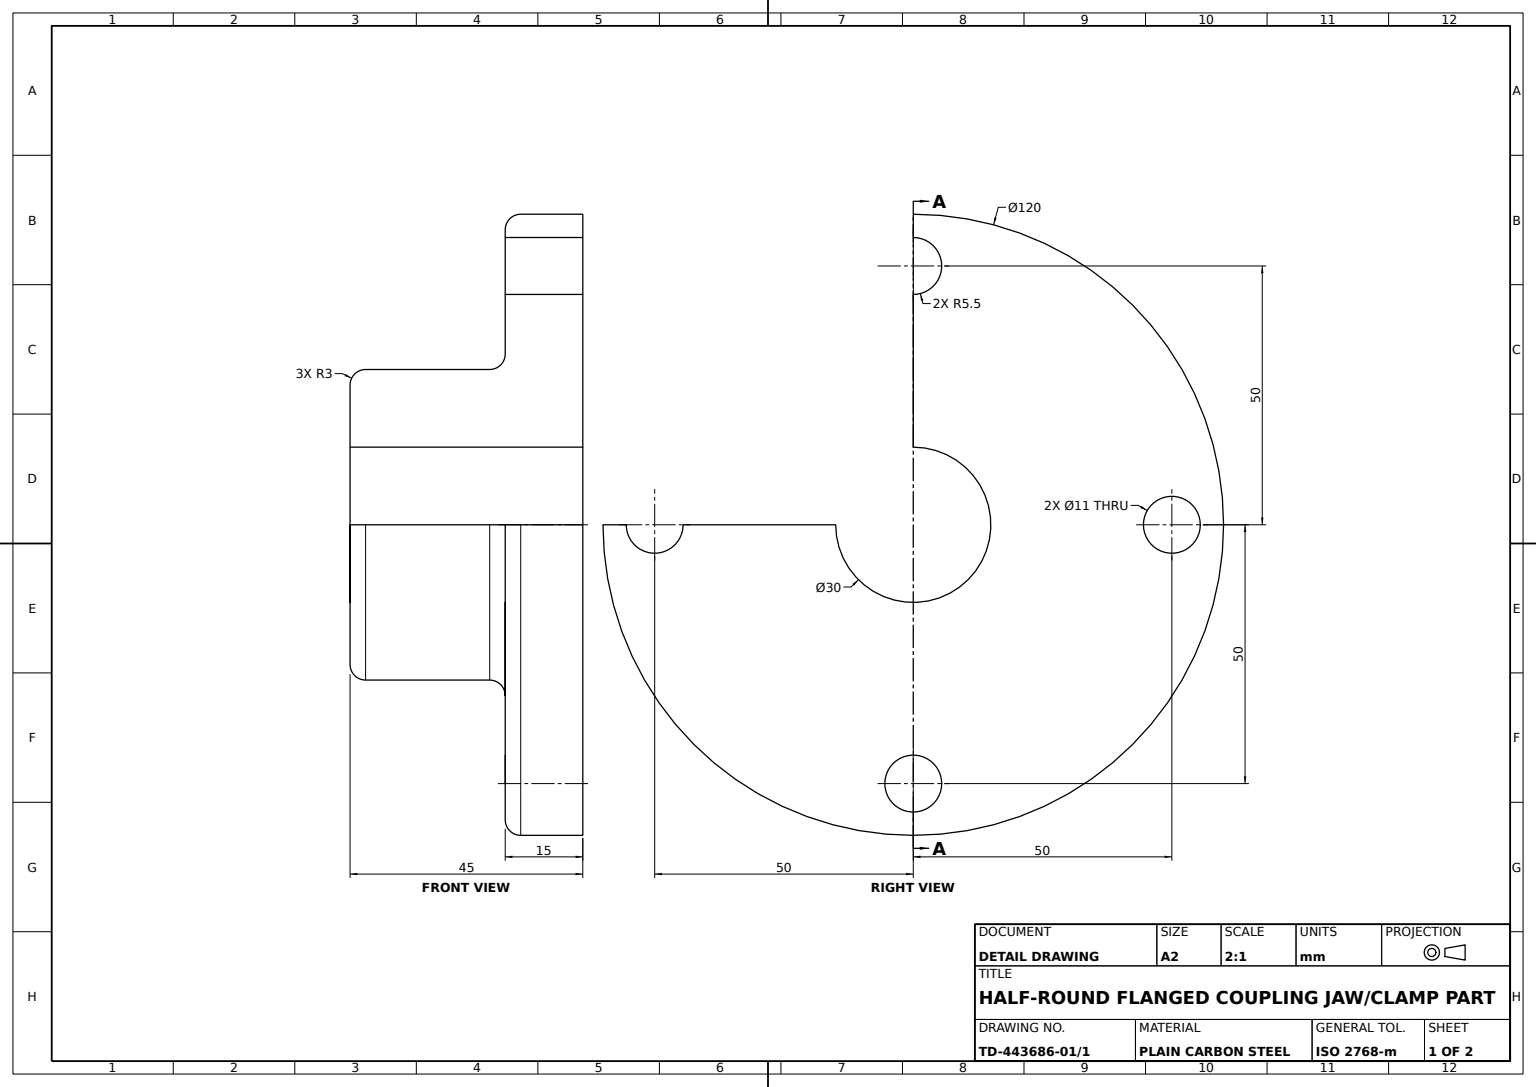
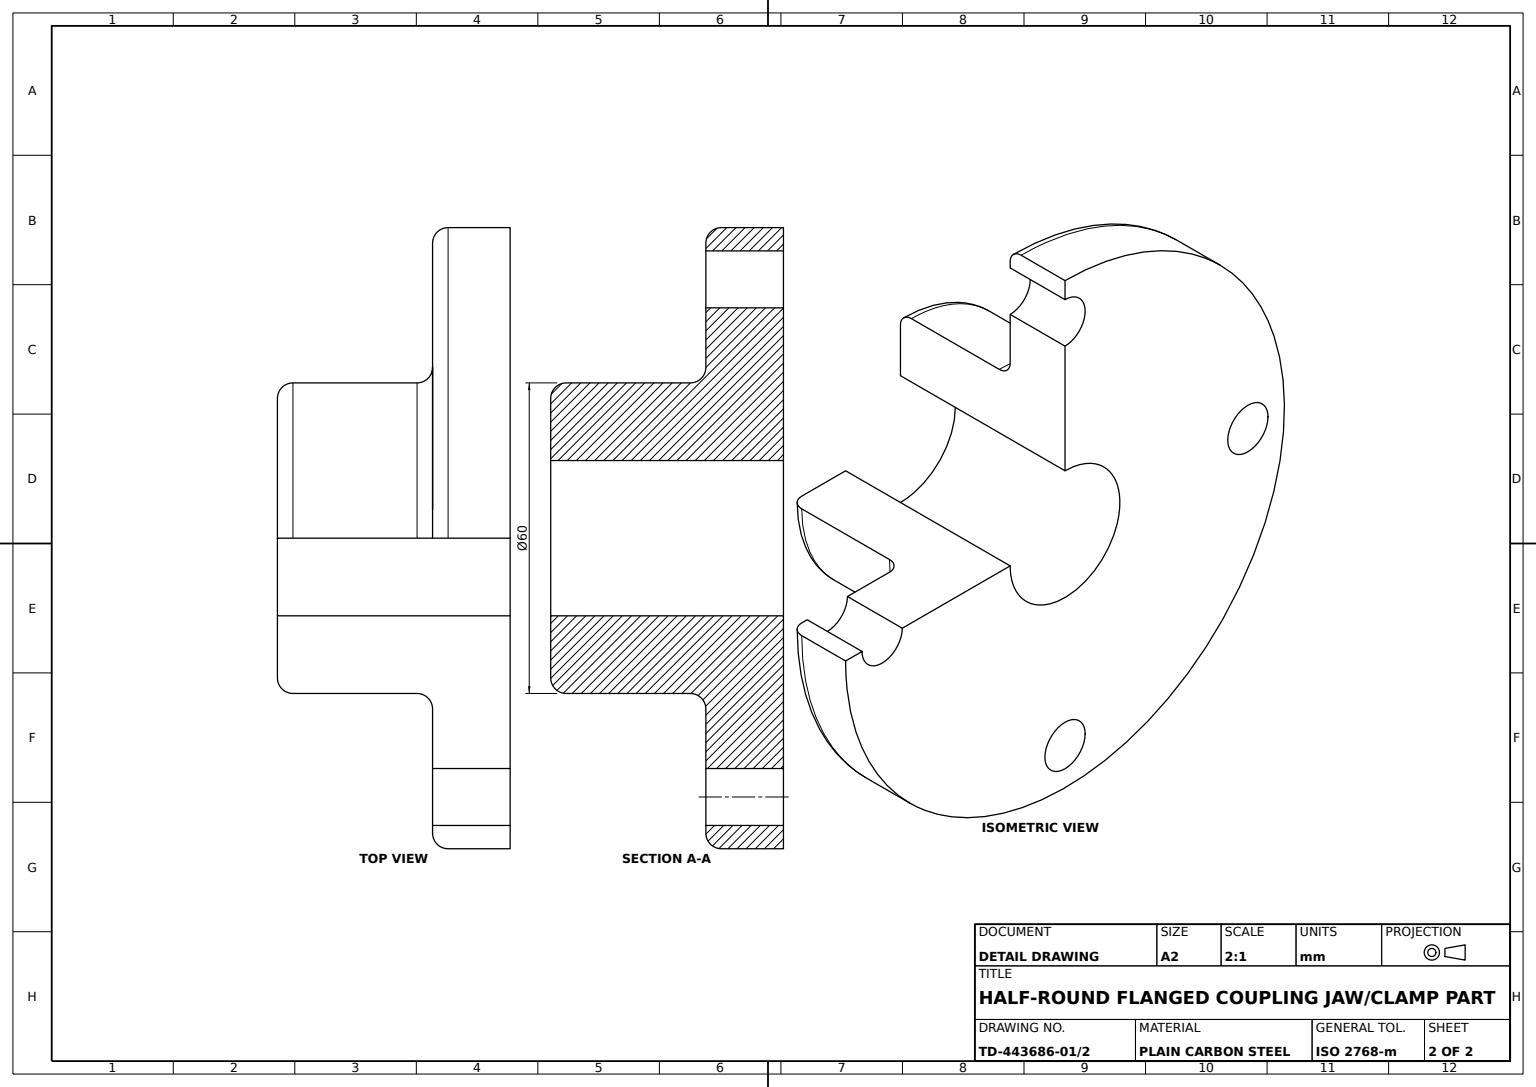
SolidWorks part; units mm, degrees
material "Plain Carbon Steel"
ref_plane "Front Plane" through (0, 0, 0) normal (0, 0, 1) x (1, 0, 0)
ref_plane "Top Plane" through (0, 0, 0) normal (0, 1, 0) x (1, 0, 0)
ref_plane "Right Plane" through (0, 0, 0) normal (1, 0, 0) x (0, 0, -1)
sketch "Bed Profile Sketch" plane through (0, 0, 0) normal (0, 0, 1) x (1, 0, 0)
  line L0 (-55.7522, 0) -> (91.5929, 0)
  line L1 (17.9204, 100.7522) -> (17.9204, -98.6283) construction
  line L2 (17.9204, 0) -> (17.9204, 15)
  line L3 (17.9204, 15) -> (-27.0796, 15)
  line L4 (-27.0796, 15) -> (-27.0796, 30)
  line L5 (-27.0796, 30) -> (2.9204, 30)
  line L6 (2.9204, 30) -> (2.9204, 60)
  line L7 (2.9204, 60) -> (17.9204, 60)
  dimension "D1" = 15
  dimension "D2" = 45
  dimension "D3" = 15
  dimension "D4" = 30
  dimension "D5" = 45
  dimension "D6" = 55.7522
  dimension "D7" = 91.5929
revolve "Bed Body Revolve" add sketch "Bed Profile Sketch" angle 360 about L0
sketch "Bolt Holes Sketch" plane through (2.9204, 0, 0) normal (-1, 0, 0) x (0, 0, 1)
  circle A0 centre (0, 0) radius 50
  circle A1 centre (0, 50) radius 5.5
  circle A2 centre (50, 0) radius 5.5
  circle A3 centre (0, -50) radius 5.5
  circle A4 centre (-50, 0) radius 5.5
  point P14 (0, 0)
  dimension "D1" = 100
  dimension "D2" = 11
  dimension "D4" = 50
  dimension "D5" = 50
  dimension "D3" = 4
extrude "Bolt Holes Ø11" cut sketch "Bolt Holes Sketch" against normal through all contours A1 | A4 | A3 | A2
fillet "Edge Fillet R3" radius 3 3 edges at (-27.0796, 0, 30) (2.9204, 0, 30) (2.9204, 0, 60)
sketch "Side Cutout Sketch" plane through (-27.0796, 0, 0) normal (-1, 0, 0) x (0, 0, 1)
  line L0 (0, 77.9575) -> (0, 0)
  line L1 (0, 0) -> (74.2223, 0)
  arc A0 (0, 77.9575) -> (74.2223, 0) centre (-1.8676, 1.8676) cw
  circle A1 centre (0, 0) radius 27 construction
  dimension "D1" = 76.1128
  dimension "D2" = 74.2223
  dimension "D3" = 1.8676
extrude "Side Cutout" cut sketch "Side Cutout Sketch" against normal through all
